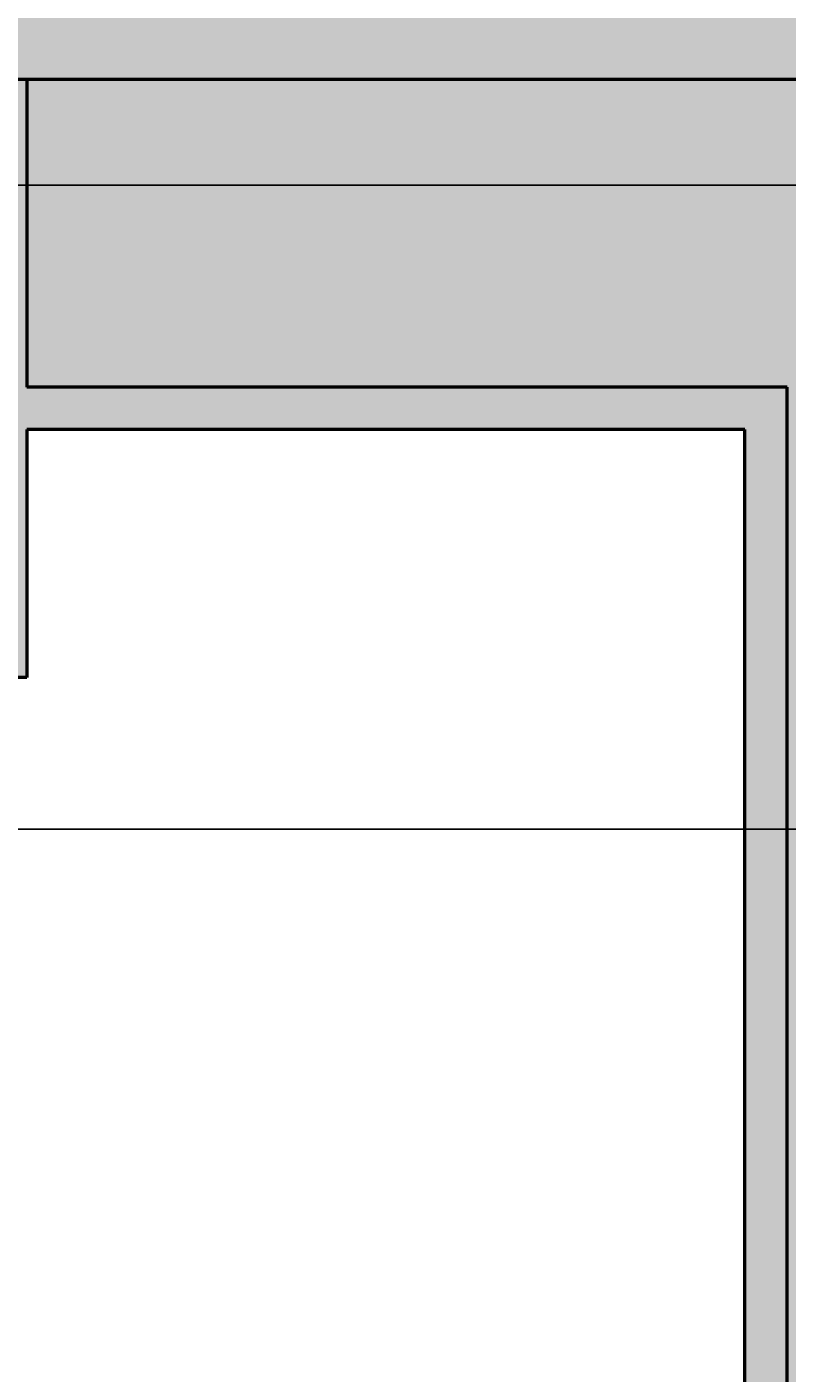
# Model space of a CAD drawing. Units: inches. Extents: x -12 to 334, y -10 to 186.
# Tile 14 of 77: x 88 to 106, y 33 to 65. Entities that reach past the tile are written whole.
import ezdxf
from ezdxf import colors
from ezdxf.entities.mleader import LeaderData, LeaderLine
from ezdxf.math import Vec2, Vec3

# ---------------------------------------------------------------- set-up
doc = ezdxf.new("R2010")
doc.units = ezdxf.units.IN
doc.header["$MEASUREMENT"] = 0
for name, color, linetype, lineweight in [('M-ANNO-TEXT', 3, 'Continuous', 25), ('M-DIMS', 2, 'Continuous', 18), ('M-EQPM', 7, 'Continuous', 50), ('M-EQPM-PATT', 8, 'Continuous', 18)]:
    doc.layers.add(name, color=color, linetype=linetype, lineweight=lineweight)
doc.styles.get("Standard").update_dxf_attribs({"font": 'arial.ttf'})
doc.dimstyles.get("Standard").update_dxf_attribs({"dimtxt": 0.18, "dimasz": 0.18, "dimexe": 0.18, "dimexo": 0.0625, "dimgap": 0.09, "dimtad": 0, "dimtih": 1, "dimtoh": 1, "dimdec": 4, "dimzin": 0, "dimdsep": 46, "dimtxsty": 'Standard', "dimcen": 0.09, "dimadec": 0, "dimazin": 0, "dimtfac": 1, "dimtdec": 4, "dimtofl": 0, "dimtmove": 0, "dimatfit": 3, "dimfxl": 1, "dimtolj": 1, "dimtzin": 0, "dimarcsym": 0})

# ---------------------------------------------------------------- blocks, each defined once
blk = doc.blocks.new('*D1')
at = {"layer": 'Defpoints', "color": 0, "transparency": 16777216}
for p in [(281.426, 91.899), (3.376, 80.692), (281.426, 14.304)]:
    blk.add_point(p, dxfattribs=at)
at = {"layer": 'M-DIMS', "color": 0, "lineweight": -2, "transparency": 16777216}
for p, q in [((281.426, 91.836), (281.426, 14.124)), ((3.376, 80.629), (3.376, 14.124)), ((3.556, 14.304), (141.935, 14.304)), ((281.246, 14.304), (142.867, 14.304))]:
    blk.add_line(p, q, dxfattribs=at)
at = {"layer": 'M-DIMS', "color": 0, "transparency": 16777216}
for points in [[(3.556, 14.334), (3.556, 14.274), (3.376, 14.304)], [(281.246, 14.334), (281.246, 14.274), (281.426, 14.304)]]:
    blk.add_solid(points, dxfattribs=at)
at = {"layer": 'M-DIMS', "color": 0, "transparency": 16777216, "insert": (142.401, 14.304), "char_height": 0.18, "attachment_point": 5}
blk.add_mtext('\\A1;278.05', dxfattribs=at)
blk = doc.blocks.new('*D29')
at = {"layer": 'Defpoints', "color": 0, "transparency": 16777216}
for p in [(-11.174, 45.854), (221.576, 45.854), (216.576, 30.854)]:
    blk.add_point(p, dxfattribs=at)
at = {"layer": 'M-DIMS', "color": 0, "lineweight": -2, "transparency": 16777216}
for p, q in [((221.514, 45.854), (-11.354, 45.854)), ((-11.174, 45.674), (-11.174, 38.536)), ((-11.174, 31.034), (-11.174, 38.172)), ((216.514, 30.854), (-11.354, 30.854))]:
    blk.add_line(p, q, dxfattribs=at)
at = {"layer": 'M-DIMS', "color": 0, "transparency": 16777216}
for points in [[(-11.204, 45.674), (-11.144, 45.674), (-11.174, 45.854)], [(-11.204, 31.034), (-11.144, 31.034), (-11.174, 30.854)]]:
    blk.add_solid(points, dxfattribs=at)
at = {"layer": 'M-DIMS', "color": 0, "transparency": 16777216, "insert": (-11.174, 38.354), "char_height": 0.18, "attachment_point": 5}
blk.add_mtext('\\A1;15', dxfattribs=at)
blk = doc.blocks.new('*D30')
at = {"layer": 'Defpoints', "color": 0, "transparency": 16777216}
for p in [(75.924, 63.612), (129.093, 61.105), (129.093, 14.304)]:
    blk.add_point(p, dxfattribs=at)
at = {"layer": 'M-DIMS', "color": 0, "lineweight": -2, "transparency": 16777216}
for p, q in [((75.924, 63.549), (75.924, 14.124)), ((129.093, 61.042), (129.093, 14.124)), ((76.104, 14.304), (102.115, 14.304)), ((128.913, 14.304), (102.902, 14.304))]:
    blk.add_line(p, q, dxfattribs=at)
at = {"layer": 'M-DIMS', "color": 0, "transparency": 16777216}
for points in [[(76.104, 14.334), (76.104, 14.274), (75.924, 14.304)], [(128.913, 14.334), (128.913, 14.274), (129.093, 14.304)]]:
    blk.add_solid(points, dxfattribs=at)
at = {"layer": 'M-DIMS', "color": 0, "transparency": 16777216, "insert": (102.509, 14.304), "char_height": 0.18, "attachment_point": 5}
blk.add_mtext('\\A1;53.17', dxfattribs=at)
blk = doc.blocks.new('*D35')
at = {"layer": 'Defpoints', "color": 0, "transparency": 16777216}
for p in [(216.428, 98.108), (-11.174, 61.105), (216.428, 61.105)]:
    blk.add_point(p, dxfattribs=at)
at = {"layer": 'M-DIMS', "color": 0, "lineweight": -2, "transparency": 16777216}
for p, q in [((216.365, 98.108), (-11.354, 98.108)), ((-11.174, 97.928), (-11.174, 79.788)), ((-11.174, 61.285), (-11.174, 79.424)), ((216.365, 61.105), (-11.354, 61.105))]:
    blk.add_line(p, q, dxfattribs=at)
at = {"layer": 'M-DIMS', "color": 0, "transparency": 16777216}
for points in [[(-11.204, 97.928), (-11.144, 97.928), (-11.174, 98.108)], [(-11.204, 61.285), (-11.144, 61.285), (-11.174, 61.105)]]:
    blk.add_solid(points, dxfattribs=at)
at = {"layer": 'M-DIMS', "color": 0, "transparency": 16777216, "insert": (-11.174, 79.606), "char_height": 0.18, "attachment_point": 5}
blk.add_mtext('\\A1;37', dxfattribs=at)
blk = doc.blocks.new('*D39')
at = {"layer": 'Defpoints', "color": 0, "transparency": 16777216}
for p in [(279.726, 80.692), (-11.174, 45.854), (269.381, 45.854)]:
    blk.add_point(p, dxfattribs=at)
at = {"layer": 'M-DIMS', "color": 0, "lineweight": -2, "transparency": 16777216}
for p, q in [((279.664, 80.692), (-11.354, 80.692)), ((-11.174, 80.512), (-11.174, 63.455)), ((-11.174, 46.034), (-11.174, 63.091)), ((269.318, 45.854), (-11.354, 45.854))]:
    blk.add_line(p, q, dxfattribs=at)
at = {"layer": 'M-DIMS', "color": 0, "transparency": 16777216}
for points in [[(-11.204, 80.512), (-11.144, 80.512), (-11.174, 80.692)], [(-11.204, 46.034), (-11.144, 46.034), (-11.174, 45.854)]]:
    blk.add_solid(points, dxfattribs=at)
at = {"layer": 'M-DIMS', "color": 0, "transparency": 16777216, "insert": (-11.174, 63.273), "char_height": 0.18, "attachment_point": 5}
blk.add_mtext('\\A1;34.84', dxfattribs=at)

msp = doc.modelspace()

# ---------------------------------------------------------------- hatches: boundary and pattern name
at = {"layer": 'M-EQPM-PATT'}
h = msp.add_hatch(color=256, dxfattribs=at)
h.set_gradient(color1=(99, 100, 102), color2=(99, 100, 102), tint=1)
h.paths.add_polyline_path([(4.3766, 80.754, -0.4132606), (23.5807, 99.8958), (37.1002, 99.8958), (37.1002, 127.7078), (32.1002, 127.7078), (32.1002, 125.2078), (36.1002, 125.2078), (36.1002, 100.8958), (23.5807, 100.8958, 1), (23.5807, 60.4872), (36.1002, 60.4872), (36.1002, 36.1752), (32.1002, 36.1752), (32.1002, 33.6752), (37.1002, 33.6752), (37.1002, 61.4872), (23.5807, 61.4872, -0.384914), (4.4744, 78.754), (72.9244, 78.754), (72.9244, 69.6117), (75.9244, 69.6117), (75.9244, 89.8963), (72.9244, 89.8963), (72.9244, 80.754)])
h.paths.add_polyline_path([(54.1002, 125.2078), (58.1002, 125.2078), (58.1002, 127.7078), (53.1002, 127.7078), (53.1002, 99.8958), (64.5, 99.8958), (64.5, 109.0583), (63.5, 109.0583), (63.5, 100.8958), (54.1002, 100.8958)], flags=17)
h.paths.add_polyline_path([(53.1002, 33.6752), (58.1002, 33.6752), (58.1002, 36.1752), (54.1002, 36.1752), (54.1002, 60.4872), (64.2068, 60.4872), (64.2068, 49.4497), (87.8879, 49.4497), (87.8879, 55.3205), (104.8919, 55.3205), (104.8919, 30.8541), (99.8919, 30.8541), (99.8919, 28.8541), (105.8919, 28.8541), (105.8919, 56.3205), (87.8879, 56.3205), (87.8879, 63.6117), (86.8879, 63.6117), (86.8879, 50.4497), (65.0061, 50.4497), (65.0061, 63.6117), (64.5, 63.6117), (64.5, 61.4872), (53.1002, 61.4872)])
h.paths.add_polyline_path([(121.8919, 28.8541), (121.8919, 30.8541), (116.8919, 30.8541), (116.8919, 45.8541), (209.6965, 45.8541), (209.9204, 46.8541), (115.8919, 46.8541), (115.8919, 28.8541)])
h.paths.add_polyline_path([(221.5761, 32.8541), (216.5761, 32.8541), (216.5761, 30.8541), (222.5761, 30.8541), (222.5761, 46.8541), (209.9204, 46.8541), (209.6965, 45.8541), (221.5761, 45.8541)])
h.paths.add_polyline_path([(233.5761, 45.8541), (249.8485, 45.8541), (249.3759, 46.8541), (232.5761, 46.8541), (232.5761, 30.8541), (238.5761, 30.8541), (238.5761, 32.8541), (233.5761, 32.8541)])
h = msp.add_hatch(color=256, dxfattribs=at)
h.set_gradient(color1=(205, 32, 39), color2=(205, 32, 39), tint=1)
h.paths.add_polyline_path([(64.5, 80.754), (64.5, 89.8963), (226.6083, 89.8963, -1), (226.6083, 69.6117), (64.5, 69.6117), (64.5, 78.754), (4.4744, 78.754, 0.384914), (23.5807, 61.4872), (37.1002, 61.4872), (37.1002, 33.6752), (53.1002, 33.6752), (53.1002, 61.4872), (64.5, 61.4872), (64.5, 63.6117), (226.6083, 63.6117, 1), (226.6083, 95.8963), (64.5, 95.8963), (64.5, 99.8958), (53.1002, 99.8958), (53.1002, 127.7078), (37.1002, 127.7078), (37.1002, 99.8958), (23.5807, 99.8958, 0.4132606), (4.3766, 80.754)])
h.paths.add_polyline_path([(64.5, 91.8963), (64.5, 93.8963), (226.6083, 93.8963, -1), (226.6083, 65.6117), (64.5, 65.6117), (64.5, 67.6117), (226.6083, 67.6117, 1), (226.6083, 91.8963)], flags=16)
h = msp.add_hatch(color=256, dxfattribs=at)
h.set_gradient(color1=(94, 103, 175), color2=(94, 103, 175), tint=1)
h.paths.add_polyline_path([(129.093, 89.8963), (86.8879, 89.8963), (86.8879, 69.6117), (129.093, 69.6117)], flags=17)
h.paths.add_polyline_path([(170.9079, 89.8963), (130.8573, 89.8963), (130.8573, 69.6117), (170.9079, 69.6117)], flags=17)
h.paths.add_polyline_path([(216.4278, 89.8963), (172.6722, 89.8963), (172.6722, 69.6117), (216.4278, 69.6117)], flags=17)
h.paths.add_polyline_path([(245.9354, 82.6969), (247.9354, 82.6969), (247.9354, 46.8541), (268.3808, 46.8541, 0.0998398), (279.7263, 80.6915), (251.9801, 80.6915, 0.4142136), (231.7758, 100.8958), (84.7229, 100.8958), (84.7229, 109.0583), (83.7229, 109.0583), (83.7229, 95.8963), (129.093, 95.8963), (129.093, 98.1081), (130.8573, 98.1081), (130.8573, 95.8963), (170.9079, 95.8963), (170.9079, 98.1081), (172.6722, 98.1081), (172.6722, 95.8963), (216.4278, 95.8963), (216.4278, 98.1081), (218.1922, 98.1081), (218.1922, 95.8963), (226.6083, 95.8963, -1), (226.6083, 63.6117), (218.1922, 63.6117), (218.1922, 61.1045), (216.4278, 61.1045), (216.4278, 63.6117), (172.6722, 63.6117), (172.6722, 61.1045), (170.9079, 61.1045), (170.9079, 63.6117), (130.8573, 63.6117), (130.8573, 61.1045), (129.093, 61.1045), (129.093, 63.6117), (87.8879, 63.6117), (87.8879, 56.3205), (105.8919, 56.3205), (105.8919, 28.8541), (115.8919, 28.8541), (115.8919, 46.8541), (222.5761, 46.8541), (222.5761, 30.8541), (232.5761, 30.8541), (232.5761, 46.8541), (245.9354, 46.8541)])
h.paths.add_polyline_path([(86.8879, 89.8963), (75.9244, 89.8963), (75.9244, 69.6117), (86.8879, 69.6117)])
h.paths.add_polyline_path([(83.7229, 109.0583), (75.9244, 109.0583), (75.9244, 95.8963), (83.7229, 95.8963)])
h.paths.add_polyline_path([(226.6083, 89.8963), (218.1922, 89.8963), (218.1922, 69.6117), (226.6083, 69.6117, 1)], flags=17)
h = msp.add_hatch(color=256, dxfattribs=at)
h.set_gradient(color1=(0, 0, 255), color2=(0, 0, 255), tint=1)
h.paths.add_polyline_path([(84.7229, 100.8958), (84.7229, 109.0583), (83.7229, 109.0583), (83.7229, 95.8963), (129.093, 95.8963), (129.093, 98.1081), (130.8573, 98.1081), (130.8573, 95.8963), (170.9079, 95.8963), (170.9079, 98.1081), (172.6722, 98.1081), (172.6722, 95.8963), (216.4278, 95.8963), (216.4278, 98.1081), (218.1922, 98.1081), (218.1922, 95.8963), (226.6083, 95.8963, -1), (226.6083, 63.6117), (218.1922, 63.6117), (218.1922, 61.1045), (216.4278, 61.1045), (216.4278, 63.6117), (172.6722, 63.6117), (172.6722, 61.1045), (170.9079, 61.1045), (170.9079, 63.6117), (130.8573, 63.6117), (130.8573, 61.1045), (129.093, 61.1045), (129.093, 63.6117), (87.8879, 63.6117), (87.8879, 56.3205), (105.8919, 56.3205), (105.8919, 28.8541), (115.8919, 28.8541), (115.8919, 46.8541), (222.5761, 46.8541), (222.5761, 30.8541), (232.5761, 30.8541), (232.5761, 46.8541), (245.9354, 46.8541), (245.9354, 82.6969), (247.9354, 82.6969), (247.9354, 46.8541), (268.3808, 46.8541, 0.0998398), (279.7263, 80.6915), (251.9801, 80.6915, 0.4142136), (231.7758, 100.8958)])

# ---------------------------------------------------------------- linework, layer by layer
at = {"layer": 'M-EQPM'}
for p, q in [((105.8919, 56.3205), (87.8879, 56.3205)), ((105.8919, 28.8541), (105.8919, 56.3205)), ((104.8919, 55.3205), (87.8879, 55.3205)), ((87.8879, 55.3205), (87.8879, 49.4497)), ((104.8919, 30.8541), (104.8919, 55.3205)), ((87.8879, 49.4497), (64.2068, 49.4497))]:
    msp.add_line(p, q, dxfattribs=at)
msp.add_lwpolyline([(64.5, 63.6117), (226.6083, 63.6117, 1), (226.6083, 95.8963), (64.5, 95.8963)], format="xyb", dxfattribs=at)
msp.add_lwpolyline([(87.8879, 63.6117), (87.8879, 56.3205)], dxfattribs=at)

# ---------------------------------------------------------------- dimensions: what is measured, and where the dimension line sits
at = {"layer": 'M-DIMS'}
for base, p1, p2, override, picture, middle in [((-11.1736, 61.1045), (216.4278, 98.1081), (216.4278, 61.1045), {"dimdec": 0, "dimlfac": 1, "dimrnd": 0, "dimzin": 0, "dimdsep": 46, "dimlunit": 2}, '*D35', (-11.1735, 79.6063)), ((-11.1736, 45.8541), (279.7263, 80.6915), (269.3808, 45.8541), {"dimdec": 2, "dimlfac": 1, "dimrnd": 0, "dimzin": 0, "dimdsep": 46, "dimlunit": 2}, '*D39', (-11.1735, 63.2728)), ((-11.1736, 45.8541), (216.5761, 30.8541), (221.5761, 45.8541), {"dimdec": 0, "dimlfac": 1, "dimrnd": 0, "dimzin": 0, "dimdsep": 46, "dimlunit": 2}, '*D29', (-11.1735, 38.3541))]:
    dim = msp.add_linear_dim(base=base, p1=p1, p2=p2, angle=90, dimstyle='Standard', override=override, dxfattribs=at)
    dim.commit()
    dim.dimension.update_dxf_attribs({"geometry": picture, "text_midpoint": middle})
for base, p1, p2, picture, middle in [((281.4256, 14.3041), (3.3765, 80.6915), (281.4256, 91.8988), '*D1', (142.401, 14.3041)), ((129.093, 14.3041), (75.9244, 63.6117), (129.093, 61.1045), '*D30', (102.5087, 14.3041))]:
    dim = msp.add_linear_dim(base=base, p1=p1, p2=p2, dimstyle='Standard', override={"dimdec": 2, "dimlfac": 1, "dimrnd": 0, "dimzin": 0, "dimdsep": 46, "dimlunit": 2}, dxfattribs=at)
    dim.commit()
    dim.dimension.update_dxf_attribs({"geometry": picture, "text_midpoint": middle})

# ---------------------------------------------------------------- leaders
at = {"layer": 'M-ANNO-TEXT'}
ml = msp.add_multileader_mtext('Standard', dxfattribs=at)
ml.set_content('^ICondensate outlet', color=256)
ml.set_leader_properties()
ml.build(insert=Vec2(0, 0))
ml.multileader.update_dxf_attribs({"dogleg_length": 0.36, "arrow_head_size": 0.7})
ctx = ml.context
ctx.base_point, ctx.arrow_head_size, ctx.landing_gap_size, ctx.plane_origin = Vec3(83.8784, 10.3512), 0.7, 0.09, Vec3(49.4251, 25.7584)
notes = []
notes.append((ctx, [(0, (1, 1, 0), (70.8242, 10.3512), (1, 0), 13.0542, [(0, [(42.9275, 33.6752)], 0, [])])]))
ctx.mtext.insert, ctx.mtext.flow_direction = Vec3(83.9684, 12.3853), 5
for ctx, leaders in notes:
    for number, flags, end, landing, length, lines in leaders:
        leader = LeaderData()
        leader.index, (leader.has_last_leader_line, leader.has_dogleg_vector, leader.attachment_direction) = number, flags
        leader.last_leader_point, leader.dogleg_vector, leader.dogleg_length = Vec3(end), Vec3(landing), length
        for number, points, colour, breaks in lines:
            line = LeaderLine()
            line.index, line.vertices, line.color, line.breaks = number, Vec3.list(points), colors.encode_raw_color(colour), breaks
            leader.lines.append(line)
        ctx.leaders.append(leader)

doc.saveas('drawing.dxf')
